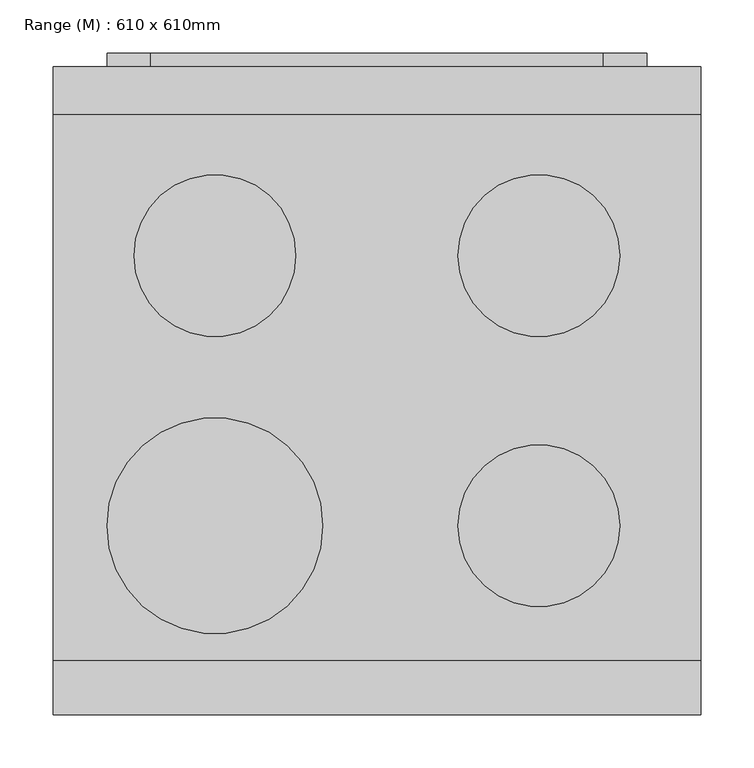
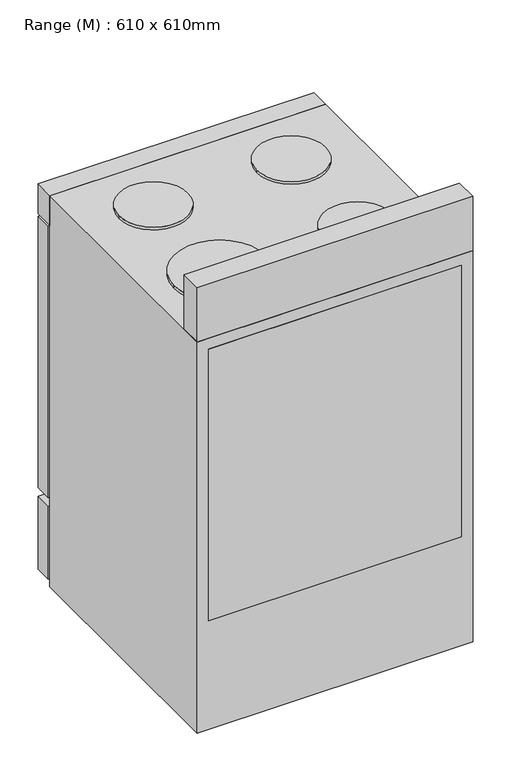
"""IFC4 building model written with IfcOpenShell, lengths in millimetres: proxy geometry, Range (M) : 610 x 610mm."""

from ifc_helpers import new_model, si_unit, point, frame, frame_2d, origin, place, context, project, spatial, polyline, circle_curve, trimmed, segment, composite_curve, outline, extrude, source, transform, mapped, element, save


def range_m_610_x_610mm_7142e668(model_context):
    return source(origin(), model_context, "Body", "SweptSolid", [
        extrude(outline(polyline([(517.925, 12.7), (517.925, 0.0), (91.687309, 0.0), (91.687309, 12.7), (517.925, 12.7)])), frame((0.0, 0.0, 791.2768639), z_axis=(0.0, 0.0, 1.0), x_axis=(1.0, 0.0, 0.0)), (0.0, 0.0, 1.0), 19.05),
        extrude(outline(polyline([(533.8, -12.7), (533.8, -19.05), (76.2, -19.05), (76.2, -12.7), (533.8, -12.7)])), frame((0.0, 0.0, 330.2), z_axis=(0.0, 0.0, 1.0), x_axis=(1.0, 0.0, 0.0)), (0.0, 0.0, 1.0), 406.4),
        extrude(outline(polyline([(610.0, 0.0), (610.0, -45.0), (0.0, -45.0), (0.0, 0.0), (610.0, 0.0)])), frame((0.0, 0.0, 844.7720355), z_axis=(0.0, 0.0, 1.0), x_axis=(1.0, 0.0, 0.0)), (0.0, 0.0, 1.0), 69.6279645),
        extrude(outline(polyline([(762.0, 559.2), (762.0, 50.8), (304.8, 50.8), (304.8, 559.2), (762.0, 559.2)]), holes=[polyline([(736.6, 533.8), (330.2, 533.8), (330.2, 76.2), (736.6, 76.2), (736.6, 533.8)])]), frame((0.0, -25.4, 0.0), z_axis=(0.0, 1.0, 0.0), x_axis=(0.0, 0.0, 1.0)), (0.0, 0.0, 1.0), 38.1),
        extrude(outline(composite_curve([segment(trimmed(circle_curve(frame_2d((152.4, -432.2)), 101.6), [point((50.8, -432.2))], [point((254.0, -432.2))], False, "CARTESIAN"), True, "CONTINUOUS"), segment(trimmed(circle_curve(frame_2d((152.4, -432.2)), 101.6), [point((254.0, -432.2))], [point((50.8, -432.2))], False, "CARTESIAN"), True, "CONTINUOUS")], self_intersect=False)), frame((0.0, 0.0, 914.4), z_axis=(0.0, 0.0, 1.0), x_axis=(1.0, 0.0, 0.0)), (0.0, 0.0, 1.0), 6.35),
        extrude(outline(composite_curve([segment(trimmed(circle_curve(frame_2d((457.6, -432.2)), 76.2), [point((381.4, -432.2))], [point((533.8, -432.2))], False, "CARTESIAN"), True, "CONTINUOUS"), segment(trimmed(circle_curve(frame_2d((457.6, -432.2)), 76.2), [point((533.8, -432.2))], [point((381.4, -432.2))], False, "CARTESIAN"), True, "CONTINUOUS")], self_intersect=False)), frame((0.0, 0.0, 914.4), z_axis=(0.0, 0.0, 1.0), x_axis=(1.0, 0.0, 0.0)), (0.0, 0.0, 1.0), 6.35),
        extrude(outline(composite_curve([segment(trimmed(circle_curve(frame_2d((457.6, -177.8)), 76.2), [point((381.4, -177.8))], [point((533.8, -177.8))], False, "CARTESIAN"), True, "CONTINUOUS"), segment(trimmed(circle_curve(frame_2d((457.6, -177.8)), 76.2), [point((533.8, -177.8))], [point((381.4, -177.8))], False, "CARTESIAN"), True, "CONTINUOUS")], self_intersect=False)), frame((0.0, 0.0, 914.4), z_axis=(0.0, 0.0, 1.0), x_axis=(1.0, 0.0, 0.0)), (0.0, 0.0, 1.0), 6.35),
        extrude(outline(composite_curve([segment(trimmed(circle_curve(frame_2d((152.4, -177.8)), 76.2), [point((76.2, -177.8))], [point((228.6, -177.8))], False, "CARTESIAN"), True, "CONTINUOUS"), segment(trimmed(circle_curve(frame_2d((152.4, -177.8)), 76.2), [point((228.6, -177.8))], [point((76.2, -177.8))], False, "CARTESIAN"), True, "CONTINUOUS")], self_intersect=False)), frame((0.0, 0.0, 914.4), z_axis=(0.0, 0.0, 1.0), x_axis=(1.0, 0.0, 0.0)), (0.0, 0.0, 1.0), 6.35),
        extrude(outline(polyline([(25.4, -610.0), (25.4, -584.6), (584.6, -584.6), (584.6, -610.0), (25.4, -610.0)])), frame((0.0, 0.0, 254.0), z_axis=(0.0, 0.0, 1.0), x_axis=(1.0, 0.0, 0.0)), (0.0, 0.0, 1.0), 635.2220355),
        extrude(outline(polyline([(838.4220355, 610.0), (838.4220355, 0.0), (203.2, 0.0), (203.2, 610.0), (838.4220355, 610.0)]), holes=[polyline([(762.0, 559.2), (304.8, 559.2), (304.8, 50.8), (762.0, 50.8), (762.0, 559.2)])]), frame((0.0, -38.1, 0.0), z_axis=(0.0, 1.0, 0.0), x_axis=(0.0, 0.0, 1.0)), (0.0, 0.0, 1.0), 38.1),
        extrude(outline(polyline([(610.0, 0.0), (610.0, -38.1), (0.0, -38.1), (0.0, 0.0), (610.0, 0.0)])), frame((0.0, 0.0, 12.7), z_axis=(0.0, 0.0, 1.0), x_axis=(1.0, 0.0, 0.0)), (0.0, 0.0, 1.0), 171.45),
        extrude(outline(polyline([(914.4, 610.0), (914.4, 0.0), (0.0, 0.0), (0.0, 610.0), (914.4, 610.0)]), holes=[polyline([(889.2220355, 584.6), (254.0, 584.6), (254.0, 25.4), (889.2220355, 25.4), (889.2220355, 584.6)])]), frame((0.0, -610.0, 0.0), z_axis=(0.0, 1.0, 0.0), x_axis=(0.0, 0.0, 1.0)), (0.0, 0.0, 1.0), 565.0),
        extrude(outline(polyline([(610.0, -610.0), (0.0, -610.0), (0.0, -559.2), (610.0, -559.2), (610.0, -610.0)])), frame((0.0, 0.0, 914.4), z_axis=(0.0, 0.0, 1.0), x_axis=(1.0, 0.0, 0.0)), (0.0, 0.0, 1.0), 127.0),
    ])


if __name__ == "__main__":
    model = new_model("IFC4")
    model_context = context("Model", 3, world=origin())
    ifc_project = project(units=[si_unit("LENGTHUNIT", "METRE", prefix="MILLI")], contexts=[model_context])
    site = spatial("IfcSite", under=ifc_project)
    building = spatial("IfcBuilding", under=site)
    placement = place(None, origin())
    range_m_610_x_610mm_shape = range_m_610_x_610mm_7142e668(model_context)
    element("IfcBuildingElementProxy", 1, Name="Range (M) : 610 x 610mm", ObjectType="Range (M) : 610 x 610mm", at=placement, inside=building, context=model_context, shape_type="MappedRepresentation", body=[
        mapped(range_m_610_x_610mm_shape, transform((0.0, 0.0, 0.0), x_axis=(1.0, 0.0, 0.0), y_axis=(0.0, 1.0, 0.0), z_axis=(0.0, 0.0, 1.0))),
    ])
    save(model, "model.ifc")

# Revit data of these elements
# Type "Range (M) : 610 x 610mm"
#   Depth = 2' - 0.01575"
#   Width = 2' - 0.01575"
#   Burner Material = Metal - Chrome
#   Range Material = Metal - Painted Finish - Ivory,Matte
#   Default Elevation = 0
#   Assembly Code = ""
# Element 1 (IfcBuildingElementProxy, "Range (M) : 610 x 610mm")
#   Materials on its faces: "Metal - Painted Finish - Ivory,Matte", "Metal - Chrome", "Glass"
# Materials
#   "Metal - Chrome": colour RGB 17 17 17, transparency 0
#   "Metal - Painted Finish - Ivory,Matte": colour RGB 247 247 239, transparency 0
#   "Glass": class "Glass", colour RGB 0 128 192, transparency 0.75, Description = "Soda Lime Glass", Cost = 0
